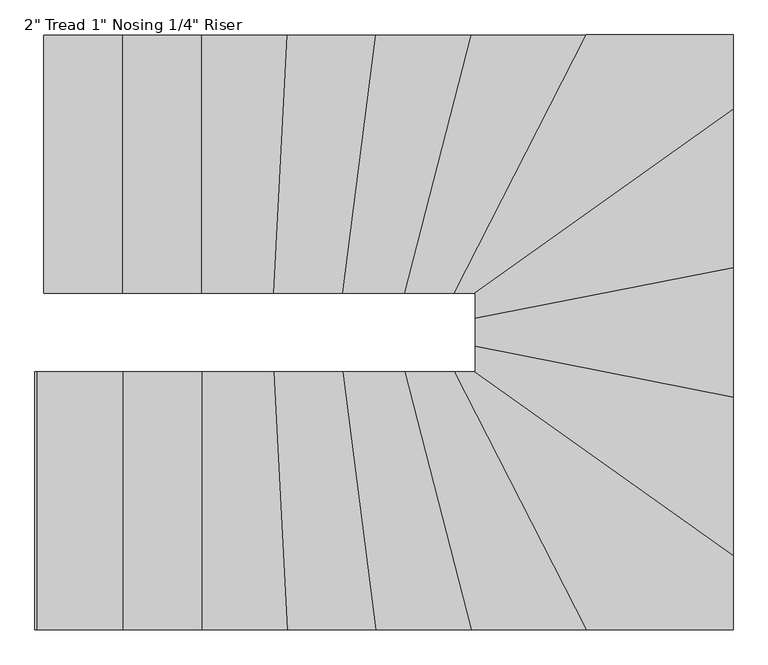
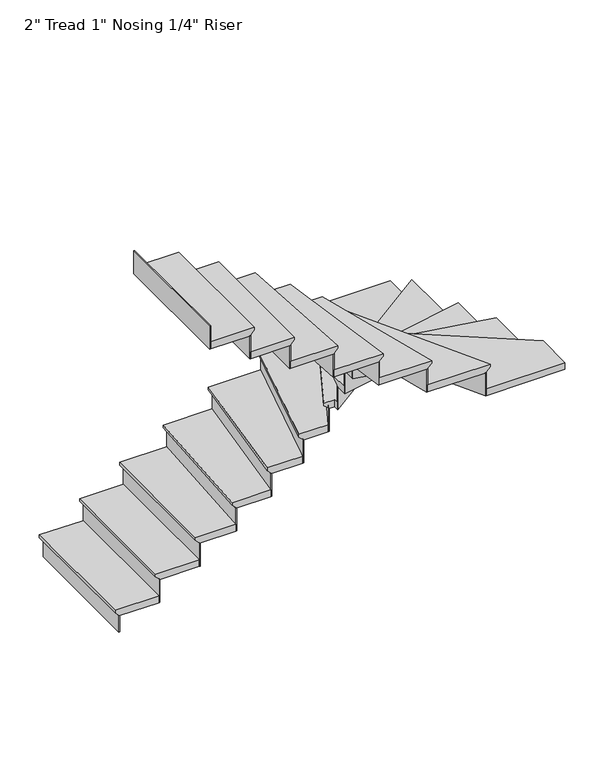
"""IFC4 building model written with IfcOpenShell, lengths in millimetres: stair flight geometry."""

from ifc_helpers import new_model, si_unit, origin, place, context, project, spatial, faceted_brep, source, transform, mapped, element, save


def stair_flight_12d8a344(model_context):
    return source(origin(), model_context, "Body", "Brep", [
        faceted_brep([(-5644.7377406, -3199.6567046, 150.2833333), (-5644.7377406, -3199.6567046, 169.3333333), (-5644.7377406, -2285.2567046, 169.3333333), (-5644.7377406, -2285.2567046, 150.2833333), (-5619.3377406, -3199.6567046, 124.8833333), (-5619.3377406, -2285.2567046, 124.8833333), (-5339.9377406, -3199.6567046, 169.3333333), (-5339.9377406, -2285.2567046, 169.3333333), (-5619.3377406, -2285.2567046, 118.5333333), (-5339.9377406, -2285.2567046, 118.5333333), (-5339.9377406, -3199.6567046, 118.5333333), (-5619.3377406, -3199.6567046, 118.5333333)], [[[0, 1, 2, 3]], [[4, 0, 3, 5]], [[2, 1, 6, 7]], [[8, 9, 10, 11]], [[2, 7, 9, 8, 5, 3]], [[8, 11, 4, 5]], [[6, 1, 0, 4, 11, 10]], [[7, 6, 10, 9]]]),
        faceted_brep([(-5619.3377406, -3199.6567046, 118.5333333), (-5619.3377406, -3199.6567046, 0.0), (-5612.9877406, -3199.6567046, 0.0), (-5612.9877406, -3199.6567046, 118.5333333), (-5619.3377406, -2285.2567046, 118.5333333), (-5612.9877406, -2285.2567046, 118.5333333), (-5612.9877406, -2285.2567046, 0.0), (-5619.3377406, -2285.2567046, 0.0)], [[[0, 1, 2, 3]], [[4, 5, 6, 7]], [[1, 0, 4, 7]], [[2, 1, 7, 6]], [[3, 2, 6, 5]], [[0, 3, 5, 4]]]),
        faceted_brep([(-5339.9377406, -3199.6567046, 287.8666667), (-5339.9377406, -3199.6567046, 118.5333333), (-5333.5877406, -3199.6567046, 118.5333333), (-5333.5877406, -3199.6567046, 287.8666667), (-5339.9377406, -2285.2567046, 287.8666667), (-5333.5877406, -2285.2567046, 287.8666667), (-5333.5877406, -2285.2567046, 118.5333333), (-5339.9377406, -2285.2567046, 118.5333333)], [[[0, 1, 2, 3]], [[4, 5, 6, 7]], [[1, 0, 4, 7]], [[2, 1, 7, 6]], [[3, 2, 6, 5]], [[0, 3, 5, 4]]]),
        faceted_brep([(-5365.3377406, -2285.2567046, 338.6666667), (-5365.3377406, -3199.6567046, 338.6666667), (-5060.5377406, -3199.6567046, 338.6666667), (-5060.5377406, -2285.2567046, 338.6666667), (-5339.9377406, -2285.2567046, 287.8666667), (-5060.5377406, -2285.2567046, 287.8666667), (-5060.5377406, -3199.6567046, 287.8666667), (-5339.9377406, -3199.6567046, 287.8666667), (-5339.9377406, -2285.2567046, 294.2166667), (-5365.3377406, -2285.2567046, 319.6166667), (-5339.9377406, -3199.6567046, 294.2166667), (-5365.3377406, -3199.6567046, 319.6166667)], [[[0, 1, 2, 3]], [[4, 5, 6, 7]], [[0, 3, 5, 4, 8, 9]], [[4, 7, 10, 8]], [[2, 1, 11, 10, 7, 6]], [[3, 2, 6, 5]], [[11, 1, 0, 9]], [[10, 11, 9, 8]]]),
        faceted_brep([(-5060.5377406, -3199.6567046, 457.2), (-5060.5377406, -3199.6567046, 287.8666667), (-5054.1877406, -3199.6567046, 287.8666667), (-5054.1877406, -3199.6567046, 457.2), (-5060.5377406, -2285.2567046, 457.2), (-5054.1877406, -2285.2567046, 457.2), (-5054.1877406, -2285.2567046, 287.8666667), (-5060.5377406, -2285.2567046, 287.8666667)], [[[0, 1, 2, 3]], [[4, 5, 6, 7]], [[1, 0, 4, 7]], [[2, 1, 7, 6]], [[3, 2, 6, 5]], [[0, 3, 5, 4]]]),
        faceted_brep([(-5085.9377406, -2285.2567046, 508.0), (-5085.9377406, -3199.6567046, 508.0), (-4804.8705791, -3199.6567046, 508.0), (-4757.3363087, -2285.2567046, 508.0), (-5060.5377406, -2285.2567046, 457.2), (-4757.3363087, -2285.2567046, 457.2), (-4804.8705791, -3199.6567046, 457.2), (-5060.5377406, -3199.6567046, 457.2), (-5060.5377406, -2285.2567046, 463.55), (-5085.9377406, -2285.2567046, 488.95), (-5060.5377406, -3199.6567046, 463.55), (-5085.9377406, -3199.6567046, 488.95)], [[[0, 1, 2, 3]], [[4, 5, 6, 7]], [[0, 3, 5, 4, 8, 9]], [[4, 7, 10, 8]], [[2, 1, 11, 10, 7, 6]], [[3, 2, 6, 5]], [[11, 1, 0, 9]], [[10, 11, 9, 8]]]),
        faceted_brep([(-4804.8705791, -3199.6567046, 626.5333333), (-4804.8705791, -3199.6567046, 457.2), (-4798.512005, -3199.6567046, 457.2), (-4798.512005, -3199.6567046, 626.5333333), (-4757.3363087, -2285.2567046, 626.5333333), (-4750.9777346, -2285.2567046, 626.5333333), (-4750.9777346, -2285.2567046, 457.2), (-4757.3363087, -2285.2567046, 457.2)], [[[0, 1, 2, 3]], [[4, 5, 6, 7]], [[1, 0, 4, 7]], [[2, 1, 7, 6]], [[3, 2, 6, 5]], [[0, 3, 5, 4]]]),
        faceted_brep([(-4782.7706054, -2285.2567046, 677.3333333), (-4830.3048758, -3199.6567046, 677.3333333), (-4560.7038793, -3199.6567046, 677.3333333), (-4442.3478276, -2285.2567046, 677.3333333), (-4757.3363087, -2285.2567046, 626.5333333), (-4442.3478276, -2285.2567046, 626.5333333), (-4560.7038793, -3199.6567046, 626.5333333), (-4804.8705791, -3199.6567046, 626.5333333), (-4757.3363087, -2285.2567046, 632.8833333), (-4782.7706054, -2285.2567046, 658.2833333), (-4804.8705791, -3199.6567046, 632.8833333), (-4830.3048758, -3199.6567046, 658.2833333)], [[[0, 1, 2, 3]], [[4, 5, 6, 7]], [[0, 3, 5, 4, 8, 9]], [[4, 7, 10, 8]], [[2, 1, 11, 10, 7, 6]], [[3, 2, 6, 5]], [[11, 1, 0, 9]], [[10, 11, 9, 8]]]),
        faceted_brep([(-4560.7038793, -3199.6567046, 795.8666667), (-4560.7038793, -3199.6567046, 626.5333333), (-4554.3009075, -3199.6567046, 626.5333333), (-4554.3009075, -3199.6567046, 795.8666667), (-4442.3478276, -2285.2567046, 795.8666667), (-4435.9448559, -2285.2567046, 795.8666667), (-4435.9448559, -2285.2567046, 626.5333333), (-4442.3478276, -2285.2567046, 626.5333333)], [[[0, 1, 2, 3]], [[4, 5, 6, 7]], [[1, 0, 4, 7]], [[2, 1, 7, 6]], [[3, 2, 6, 5]], [[0, 3, 5, 4]]]),
        faceted_brep([(-4467.9597148, -2285.2567046, 846.6666667), (-4586.3157664, -3199.6567046, 846.6666667), (-4339.0766568, -3199.6567046, 846.6666667), (-4103.9462094, -2285.2567046, 846.6666667), (-4442.3478276, -2285.2567046, 795.8666667), (-4103.9462094, -2285.2567046, 795.8666667), (-4339.0766568, -3199.6567046, 795.8666667), (-4560.7038793, -3199.6567046, 795.8666667), (-4442.3478276, -2285.2567046, 802.2166667), (-4467.9597148, -2285.2567046, 827.6166667), (-4560.7038793, -3199.6567046, 802.2166667), (-4586.3157664, -3199.6567046, 827.6166667)], [[[0, 1, 2, 3]], [[4, 5, 6, 7]], [[0, 3, 5, 4, 8, 9]], [[4, 7, 10, 8]], [[2, 1, 11, 10, 7, 6]], [[3, 2, 6, 5]], [[11, 1, 0, 9]], [[10, 11, 9, 8]]]),
        faceted_brep([(-4339.0766568, -3199.6567046, 965.2), (-4339.0766568, -3199.6567046, 795.8666667), (-4332.52008, -3199.6567046, 795.8666667), (-4332.52008, -3199.6567046, 965.2), (-4103.9462094, -2285.2567046, 965.2), (-4097.3896326, -2285.2567046, 965.2), (-4097.3896326, -2285.2567046, 795.8666667), (-4103.9462094, -2285.2567046, 795.8666667)], [[[0, 1, 2, 3]], [[4, 5, 6, 7]], [[1, 0, 4, 7]], [[2, 1, 7, 6]], [[3, 2, 6, 5]], [[0, 3, 5, 4]]]),
        faceted_brep([(-4130.1725169, -2285.2567046, 1016.0), (-4365.3029643, -3199.6567046, 1016.0), (-4162.7300207, -3199.6567046, 1016.0), (-3693.9053994, -2285.2567046, 1016.0), (-4103.9462094, -2285.2567046, 965.2), (-3693.9053994, -2285.2567046, 965.2), (-4162.7300207, -3199.6567046, 965.2), (-4339.0766568, -3199.6567046, 965.2), (-4103.9462094, -2285.2567046, 971.55), (-4130.1725169, -2285.2567046, 996.95), (-4339.0766568, -3199.6567046, 971.55), (-4365.3029643, -3199.6567046, 996.95)], [[[0, 1, 2, 3]], [[4, 5, 6, 7]], [[0, 3, 5, 4, 8, 9]], [[4, 7, 10, 8]], [[2, 1, 11, 10, 7, 6]], [[3, 2, 6, 5]], [[11, 1, 0, 9]], [[10, 11, 9, 8]]]),
        faceted_brep([(-4162.7300207, -3199.6567046, 1134.5333333), (-4162.7300207, -3199.6567046, 965.2), (-4155.5940376, -3199.6567046, 965.2), (-4155.5940376, -3199.6567046, 1134.5333333), (-3693.9053994, -2285.2567046, 1134.5333333), (-3686.7694163, -2285.2567046, 1134.5333333), (-3686.7694163, -2285.2567046, 965.2), (-3693.9053994, -2285.2567046, 965.2)], [[[0, 1, 2, 3]], [[4, 5, 6, 7]], [[1, 0, 4, 7]], [[2, 1, 7, 6]], [[3, 2, 6, 5]], [[0, 3, 5, 4]]]),
        faceted_brep([(-3202.6060487, -2578.9378382, 1185.3333333), (-3202.6060487, -2285.2567046, 1185.3333333), (-3722.449332, -2285.2567046, 1185.3333333), (-4191.2739533, -3199.6567046, 1185.3333333), (-4117.0060487, -3199.6567046, 1185.3333333), (-4117.0060487, -3229.2117874, 1185.3333333), (-3202.6060487, -2285.2567046, 1134.5333333), (-3202.6060487, -2578.9378382, 1134.5333333), (-4117.0060487, -3229.2117874, 1134.5333333), (-4117.0060487, -3199.6567046, 1134.5333333), (-4162.7300207, -3199.6567046, 1134.5333333), (-3693.9053994, -2285.2567046, 1134.5333333), (-3693.9053994, -2285.2567046, 1140.8833333), (-3722.449332, -2285.2567046, 1166.2833333), (-4162.7300207, -3199.6567046, 1140.8833333), (-4191.2739533, -3199.6567046, 1166.2833333)], [[[0, 1, 2, 3, 4, 5]], [[6, 7, 8, 9, 10, 11]], [[1, 0, 7, 6]], [[2, 1, 6, 11, 12, 13]], [[11, 10, 14, 12]], [[4, 3, 15, 14, 10, 9]], [[5, 4, 9, 8]], [[0, 5, 8, 7]], [[15, 3, 2, 13]], [[14, 15, 13, 12]]]),
        faceted_brep([(-4117.0060487, -3229.2117874, 1303.8666667), (-4117.0060487, -3229.2117874, 1134.5333333), (-4117.0060487, -3237.0037622, 1134.5333333), (-4117.0060487, -3237.0037622, 1303.8666667), (-3202.6060487, -2578.9378382, 1303.8666667), (-3202.6060487, -2586.729813, 1303.8666667), (-3202.6060487, -2586.729813, 1134.5333333), (-3202.6060487, -2578.9378382, 1134.5333333)], [[[0, 1, 2, 3]], [[4, 5, 6, 7]], [[1, 0, 4, 7]], [[2, 1, 7, 6]], [[3, 2, 6, 5]], [[0, 3, 5, 4]]]),
        faceted_brep([(-3202.6060487, -2547.7699391, 1354.6666667), (-4117.0060487, -3198.0438882, 1354.6666667), (-4117.0060487, -3315.6658745, 1354.6666667), (-3202.6060487, -3135.4250181, 1354.6666667), (-3202.6060487, -2578.9378382, 1303.8666667), (-3202.6060487, -3135.4250181, 1303.8666667), (-4117.0060487, -3315.6658745, 1303.8666667), (-4117.0060487, -3229.2117874, 1303.8666667), (-3202.6060487, -2578.9378382, 1310.2166667), (-3202.6060487, -2547.7699391, 1335.6166667), (-4117.0060487, -3229.2117874, 1310.2166667), (-4117.0060487, -3198.0438882, 1335.6166667)], [[[0, 1, 2, 3]], [[4, 5, 6, 7]], [[0, 3, 5, 4, 8, 9]], [[4, 7, 10, 8]], [[2, 1, 11, 10, 7, 6]], [[3, 2, 6, 5]], [[11, 1, 0, 9]], [[10, 11, 9, 8]]]),
        faceted_brep([(-4117.0060487, -3315.6658745, 1473.2), (-4117.0060487, -3315.6658745, 1303.8666667), (-4117.0060487, -3322.1380599, 1303.8666667), (-4117.0060487, -3322.1380599, 1473.2), (-3202.6060487, -3135.4250181, 1473.2), (-3202.6060487, -3141.8972036, 1473.2), (-3202.6060487, -3141.8972036, 1303.8666667), (-3202.6060487, -3135.4250181, 1303.8666667)], [[[0, 1, 2, 3]], [[4, 5, 6, 7]], [[1, 0, 4, 7]], [[2, 1, 7, 6]], [[3, 2, 6, 5]], [[0, 3, 5, 4]]]),
        faceted_brep([(-3202.6060487, -3109.5362764, 1524.0), (-4117.0060487, -3289.7771327, 1524.0), (-4117.0060487, -3414.8250181, 1524.0), (-3202.6060487, -3595.0658745, 1524.0), (-3202.6060487, -3135.4250181, 1473.2), (-3202.6060487, -3595.0658745, 1473.2), (-4117.0060487, -3414.8250181, 1473.2), (-4117.0060487, -3315.6658745, 1473.2), (-3202.6060487, -3135.4250181, 1479.55), (-3202.6060487, -3109.5362764, 1504.95), (-4117.0060487, -3315.6658745, 1479.55), (-4117.0060487, -3289.7771327, 1504.95)], [[[0, 1, 2, 3]], [[4, 5, 6, 7]], [[0, 3, 5, 4, 8, 9]], [[4, 7, 10, 8]], [[2, 1, 11, 10, 7, 6]], [[3, 2, 6, 5]], [[11, 1, 0, 9]], [[10, 11, 9, 8]]]),
        faceted_brep([(-4117.0060487, -3414.8250181, 1642.5333333), (-4117.0060487, -3414.8250181, 1473.2), (-4117.0060487, -3421.2972036, 1473.2), (-4117.0060487, -3421.2972036, 1642.5333333), (-3202.6060487, -3595.0658745, 1642.5333333), (-3202.6060487, -3601.5380599, 1642.5333333), (-3202.6060487, -3601.5380599, 1473.2), (-3202.6060487, -3595.0658745, 1473.2)], [[[0, 1, 2, 3]], [[4, 5, 6, 7]], [[1, 0, 4, 7]], [[2, 1, 7, 6]], [[3, 2, 6, 5]], [[0, 3, 5, 4]]]),
        faceted_brep([(-3202.6060487, -3569.1771327, 1693.3333333), (-4117.0060487, -3388.9362764, 1693.3333333), (-4117.0060487, -3479.0567046, 1693.3333333), (-4163.1015233, -3479.0567046, 1693.3333333), (-3202.6060487, -4162.1113692, 1693.3333333), (-3202.6060487, -3595.0658745, 1642.5333333), (-3202.6060487, -4162.1113692, 1642.5333333), (-4163.1015233, -3479.0567046, 1642.5333333), (-4117.0060487, -3479.0567046, 1642.5333333), (-4117.0060487, -3414.8250181, 1642.5333333), (-3202.6060487, -3595.0658745, 1648.8833333), (-3202.6060487, -3569.1771327, 1674.2833333), (-4117.0060487, -3414.8250181, 1648.8833333), (-4117.0060487, -3388.9362764, 1674.2833333)], [[[0, 1, 2, 3, 4]], [[5, 6, 7, 8, 9]], [[0, 4, 6, 5, 10, 11]], [[5, 9, 12, 10]], [[2, 1, 13, 12, 9, 8]], [[3, 2, 8, 7]], [[4, 3, 7, 6]], [[13, 1, 0, 11]], [[12, 13, 11, 10]]]),
        faceted_brep([(-4163.1015233, -3479.0567046, 1811.8666667), (-4163.1015233, -3479.0567046, 1642.5333333), (-4174.0584157, -3479.0567046, 1642.5333333), (-4174.0584157, -3479.0567046, 1811.8666667), (-3202.6060487, -4162.1113692, 1811.8666667), (-3202.6060487, -4169.903344, 1811.8666667), (-3202.6060487, -4169.903344, 1642.5333333), (-3202.6060487, -4162.1113692, 1642.5333333)], [[[0, 1, 2, 3]], [[4, 5, 6, 7]], [[1, 0, 4, 7]], [[2, 1, 7, 6]], [[3, 2, 6, 5]], [[0, 3, 5, 4]]]),
        faceted_brep([(-3750.9932645, -4393.4567046, 1862.6666667), (-3202.6060487, -4393.4567046, 1862.6666667), (-3202.6060487, -4130.94347, 1862.6666667), (-4119.2739533, -3479.0567046, 1862.6666667), (-4219.8178858, -3479.0567046, 1862.6666667), (-3202.6060487, -4393.4567046, 1811.8666667), (-3750.9932645, -4393.4567046, 1811.8666667), (-4219.8178858, -3479.0567046, 1811.8666667), (-4163.1015233, -3479.0567046, 1811.8666667), (-3202.6060487, -4162.1113692, 1811.8666667), (-3202.6060487, -4162.1113692, 1818.2166667), (-3202.6060487, -4130.94347, 1843.6166667), (-4163.1015233, -3479.0567046, 1818.2166667), (-4119.2739533, -3479.0567046, 1843.6166667)], [[[0, 1, 2, 3, 4]], [[5, 6, 7, 8, 9]], [[1, 0, 6, 5]], [[2, 1, 5, 9, 10, 11]], [[9, 8, 12, 10]], [[4, 3, 13, 12, 8, 7]], [[0, 4, 7, 6]], [[13, 3, 2, 11]], [[12, 13, 11, 10]]]),
        faceted_brep([(-4219.8178858, -3479.0567046, 1981.2), (-4219.8178858, -3479.0567046, 1811.8666667), (-4226.953869, -3479.0567046, 1811.8666667), (-4226.953869, -3479.0567046, 1981.2), (-3750.9932645, -4393.4567046, 1981.2), (-3758.1292476, -4393.4567046, 1981.2), (-3758.1292476, -4393.4567046, 1811.8666667), (-3750.9932645, -4393.4567046, 1811.8666667)], [[[0, 1, 2, 3]], [[4, 5, 6, 7]], [[1, 0, 4, 7]], [[2, 1, 7, 6]], [[3, 2, 6, 5]], [[0, 3, 5, 4]]]),
        faceted_brep([(-3722.449332, -4393.4567046, 2032.0), (-4191.2739533, -3479.0567046, 2032.0), (-4391.5292718, -3479.0567046, 2032.0), (-4156.3988244, -4393.4567046, 2032.0), (-3750.9932645, -4393.4567046, 1981.2), (-4156.3988244, -4393.4567046, 1981.2), (-4391.5292718, -3479.0567046, 1981.2), (-4219.8178858, -3479.0567046, 1981.2), (-3750.9932645, -4393.4567046, 1987.55), (-3722.449332, -4393.4567046, 2012.95), (-4219.8178858, -3479.0567046, 1987.55), (-4191.2739533, -3479.0567046, 2012.95)], [[[0, 1, 2, 3]], [[4, 5, 6, 7]], [[0, 3, 5, 4, 8, 9]], [[4, 7, 10, 8]], [[2, 1, 11, 10, 7, 6]], [[3, 2, 6, 5]], [[11, 1, 0, 9]], [[10, 11, 9, 8]]]),
        faceted_brep([(-4391.5292718, -3479.0567046, 2150.5333333), (-4391.5292718, -3479.0567046, 1981.2), (-4398.0858486, -3479.0567046, 1981.2), (-4398.0858486, -3479.0567046, 2150.5333333), (-4156.3988244, -4393.4567046, 2150.5333333), (-4162.9554012, -4393.4567046, 2150.5333333), (-4162.9554012, -4393.4567046, 1981.2), (-4156.3988244, -4393.4567046, 1981.2)], [[[0, 1, 2, 3]], [[4, 5, 6, 7]], [[1, 0, 4, 7]], [[2, 1, 7, 6]], [[3, 2, 6, 5]], [[0, 3, 5, 4]]]),
        faceted_brep([(-4130.1725169, -4393.4567046, 2201.3333333), (-4365.3029643, -3479.0567046, 2201.3333333), (-4611.9276535, -3479.0567046, 2201.3333333), (-4493.5716019, -4393.4567046, 2201.3333333), (-4156.3988244, -4393.4567046, 2150.5333333), (-4493.5716019, -4393.4567046, 2150.5333333), (-4611.9276535, -3479.0567046, 2150.5333333), (-4391.5292718, -3479.0567046, 2150.5333333), (-4156.3988244, -4393.4567046, 2156.8833333), (-4130.1725169, -4393.4567046, 2182.2833333), (-4391.5292718, -3479.0567046, 2156.8833333), (-4365.3029643, -3479.0567046, 2182.2833333)], [[[0, 1, 2, 3]], [[4, 5, 6, 7]], [[0, 3, 5, 4, 8, 9]], [[4, 7, 10, 8]], [[2, 1, 11, 10, 7, 6]], [[3, 2, 6, 5]], [[11, 1, 0, 9]], [[10, 11, 9, 8]]]),
        faceted_brep([(-4611.9276535, -3479.0567046, 2319.8666667), (-4611.9276535, -3479.0567046, 2150.5333333), (-4618.3306253, -3479.0567046, 2150.5333333), (-4618.3306253, -3479.0567046, 2319.8666667), (-4493.5716019, -4393.4567046, 2319.8666667), (-4499.9745737, -4393.4567046, 2319.8666667), (-4499.9745737, -4393.4567046, 2150.5333333), (-4493.5716019, -4393.4567046, 2150.5333333)], [[[0, 1, 2, 3]], [[4, 5, 6, 7]], [[1, 0, 4, 7]], [[2, 1, 7, 6]], [[3, 2, 6, 5]], [[0, 3, 5, 4]]]),
        faceted_brep([(-4467.9597148, -4393.4567046, 2370.6666667), (-4586.3157664, -3479.0567046, 2370.6666667), (-4855.7391725, -3479.0567046, 2370.6666667), (-4808.204902, -4393.4567046, 2370.6666667), (-4493.5716019, -4393.4567046, 2319.8666667), (-4808.204902, -4393.4567046, 2319.8666667), (-4855.7391725, -3479.0567046, 2319.8666667), (-4611.9276535, -3479.0567046, 2319.8666667), (-4493.5716019, -4393.4567046, 2326.2166667), (-4467.9597148, -4393.4567046, 2351.6166667), (-4611.9276535, -3479.0567046, 2326.2166667), (-4586.3157664, -3479.0567046, 2351.6166667)], [[[0, 1, 2, 3]], [[4, 5, 6, 7]], [[0, 3, 5, 4, 8, 9]], [[4, 7, 10, 8]], [[2, 1, 11, 10, 7, 6]], [[3, 2, 6, 5]], [[11, 1, 0, 9]], [[10, 11, 9, 8]]]),
        faceted_brep([(-4855.7391725, -3479.0567046, 2489.2), (-4855.7391725, -3479.0567046, 2319.8666667), (-4862.0977466, -3479.0567046, 2319.8666667), (-4862.0977466, -3479.0567046, 2489.2), (-4808.204902, -4393.4567046, 2489.2), (-4814.5634762, -4393.4567046, 2489.2), (-4814.5634762, -4393.4567046, 2319.8666667), (-4808.204902, -4393.4567046, 2319.8666667)], [[[0, 1, 2, 3]], [[4, 5, 6, 7]], [[1, 0, 4, 7]], [[2, 1, 7, 6]], [[3, 2, 6, 5]], [[0, 3, 5, 4]]]),
        faceted_brep([(-4782.7706054, -4393.4567046, 2540.0), (-4830.3048758, -3479.0567046, 2540.0), (-5111.3377406, -3479.0567046, 2540.0), (-5111.3377406, -4393.4567046, 2540.0), (-4808.204902, -4393.4567046, 2489.2), (-5111.3377406, -4393.4567046, 2489.2), (-5111.3377406, -3479.0567046, 2489.2), (-4855.7391725, -3479.0567046, 2489.2), (-4808.204902, -4393.4567046, 2495.55), (-4782.7706054, -4393.4567046, 2520.95), (-4855.7391725, -3479.0567046, 2495.55), (-4830.3048758, -3479.0567046, 2520.95)], [[[0, 1, 2, 3]], [[4, 5, 6, 7]], [[0, 3, 5, 4, 8, 9]], [[4, 7, 10, 8]], [[2, 1, 11, 10, 7, 6]], [[3, 2, 6, 5]], [[11, 1, 0, 9]], [[10, 11, 9, 8]]]),
        faceted_brep([(-5111.3377406, -3479.0567046, 2658.5333333), (-5111.3377406, -3479.0567046, 2489.2), (-5117.6877406, -3479.0567046, 2489.2), (-5117.6877406, -3479.0567046, 2658.5333333), (-5111.3377406, -4393.4567046, 2658.5333333), (-5117.6877406, -4393.4567046, 2658.5333333), (-5117.6877406, -4393.4567046, 2489.2), (-5111.3377406, -4393.4567046, 2489.2)], [[[0, 1, 2, 3]], [[4, 5, 6, 7]], [[1, 0, 4, 7]], [[2, 1, 7, 6]], [[3, 2, 6, 5]], [[0, 3, 5, 4]]]),
        faceted_brep([(-5085.9377406, -4393.4567046, 2709.3333333), (-5085.9377406, -3479.0567046, 2709.3333333), (-5390.7377406, -3479.0567046, 2709.3333333), (-5390.7377406, -4393.4567046, 2709.3333333), (-5111.3377406, -4393.4567046, 2658.5333333), (-5390.7377406, -4393.4567046, 2658.5333333), (-5390.7377406, -3479.0567046, 2658.5333333), (-5111.3377406, -3479.0567046, 2658.5333333), (-5111.3377406, -4393.4567046, 2664.8833333), (-5085.9377406, -4393.4567046, 2690.2833333), (-5111.3377406, -3479.0567046, 2664.8833333), (-5085.9377406, -3479.0567046, 2690.2833333)], [[[0, 1, 2, 3]], [[4, 5, 6, 7]], [[0, 3, 5, 4, 8, 9]], [[4, 7, 10, 8]], [[2, 1, 11, 10, 7, 6]], [[3, 2, 6, 5]], [[11, 1, 0, 9]], [[10, 11, 9, 8]]]),
        faceted_brep([(-5390.7377406, -3479.0567046, 2827.8666667), (-5390.7377406, -3479.0567046, 2658.5333333), (-5397.0877406, -3479.0567046, 2658.5333333), (-5397.0877406, -3479.0567046, 2827.8666667), (-5390.7377406, -4393.4567046, 2827.8666667), (-5397.0877406, -4393.4567046, 2827.8666667), (-5397.0877406, -4393.4567046, 2658.5333333), (-5390.7377406, -4393.4567046, 2658.5333333)], [[[0, 1, 2, 3]], [[4, 5, 6, 7]], [[1, 0, 4, 7]], [[2, 1, 7, 6]], [[3, 2, 6, 5]], [[0, 3, 5, 4]]]),
        faceted_brep([(-5670.1377406, -3479.0567046, 2997.2), (-5670.1377406, -3479.0567046, 2827.8666667), (-5676.4877406, -3479.0567046, 2827.8666667), (-5676.4877406, -3479.0567046, 2997.2), (-5670.1377406, -4393.4567046, 2997.2), (-5676.4877406, -4393.4567046, 2997.2), (-5676.4877406, -4393.4567046, 2827.8666667), (-5670.1377406, -4393.4567046, 2827.8666667)], [[[0, 1, 2, 3]], [[4, 5, 6, 7]], [[1, 0, 4, 7]], [[2, 1, 7, 6]], [[3, 2, 6, 5]], [[0, 3, 5, 4]]]),
        faceted_brep([(-5365.3377406, -4393.4567046, 2878.6666667), (-5365.3377406, -3479.0567046, 2878.6666667), (-5670.1377406, -3479.0567046, 2878.6666667), (-5670.1377406, -4393.4567046, 2878.6666667), (-5390.7377406, -4393.4567046, 2827.8666667), (-5670.1377406, -4393.4567046, 2827.8666667), (-5670.1377406, -3479.0567046, 2827.8666667), (-5390.7377406, -3479.0567046, 2827.8666667), (-5390.7377406, -4393.4567046, 2834.2166667), (-5365.3377406, -4393.4567046, 2859.6166667), (-5390.7377406, -3479.0567046, 2834.2166667), (-5365.3377406, -3479.0567046, 2859.6166667)], [[[0, 1, 2, 3]], [[4, 5, 6, 7]], [[0, 3, 5, 4, 8, 9]], [[4, 7, 10, 8]], [[2, 1, 11, 10, 7, 6]], [[3, 2, 6, 5]], [[11, 1, 0, 9]], [[10, 11, 9, 8]]]),
    ])


if __name__ == "__main__":
    model = new_model("IFC4")
    model_context = context("Model", 3, world=origin())
    ifc_project = project(units=[si_unit("LENGTHUNIT", "METRE", prefix="MILLI")], contexts=[model_context])
    site = spatial("IfcSite", under=ifc_project)
    building = spatial("IfcBuilding", under=site)
    placement = place(None, origin())
    stair_flight_shape = stair_flight_12d8a344(model_context)
    element("IfcStairFlight", 1, ObjectType="2\" Tread 1\" Nosing 1/4\" Riser", at=placement, inside=building, context=model_context, shape_type="MappedRepresentation", body=[
        mapped(stair_flight_shape, transform((0.0, 0.0, 0.0), x_axis=(1.0, 0.0, 0.0), y_axis=(0.0, 1.0, 0.0), z_axis=(0.0, 0.0, 1.0))),
    ])
    save(model, "model.ifc")
